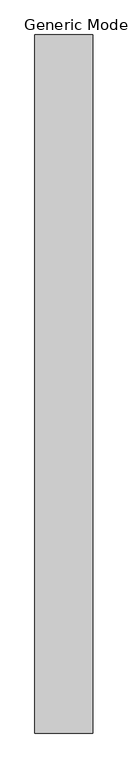
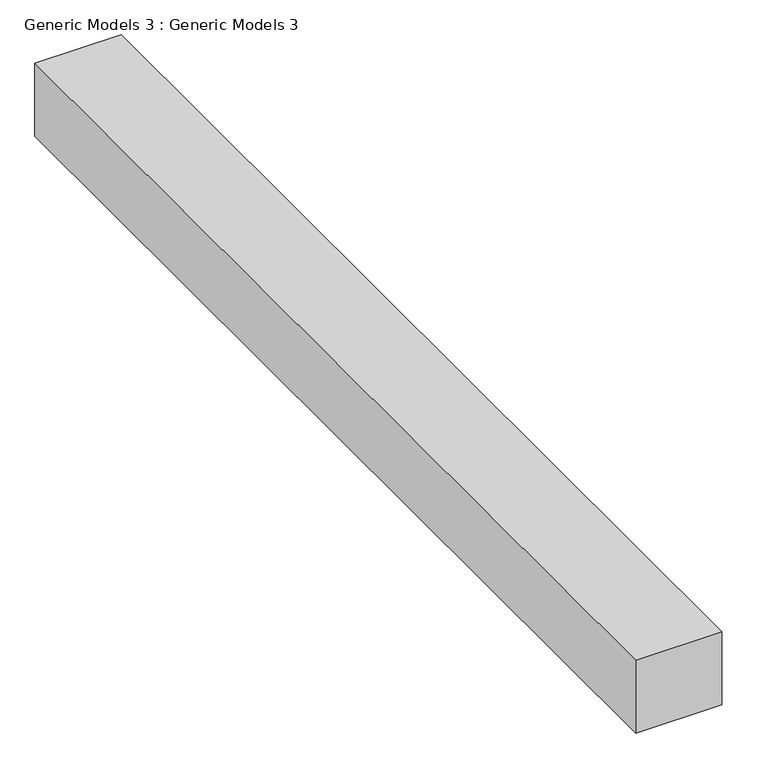
"""IFC4 building model written with IfcOpenShell, lengths in millimetres: proxy geometry, Generic Models 3 : Generic Models 3."""

from ifc_helpers import new_model, si_unit, frame, origin, place, context, project, spatial, polyline, outline, extrude, source, transform, mapped, element, save


def generic_models_3_generic_models_3_7314e451(model_context):
    return source(origin(), model_context, "Body", "SweptSolid", [
        extrude(outline(polyline([(-8586.8607234, -9739.3538163), (-8245.991855, -9739.3538163), (-8245.991855, -13854.1538163), (-8586.8607234, -13854.1538163), (-8586.8607234, -9739.3538163)])), frame((0.0, 0.0, 3352.8), z_axis=(0.0, 0.0, 1.0), x_axis=(1.0, 0.0, 0.0)), (0.0, 0.0, 1.0), 304.8),
    ])


if __name__ == "__main__":
    model = new_model("IFC4")
    model_context = context("Model", 3, world=origin())
    ifc_project = project(units=[si_unit("LENGTHUNIT", "METRE", prefix="MILLI")], contexts=[model_context])
    site = spatial("IfcSite", under=ifc_project)
    building = spatial("IfcBuilding", under=site)
    placement = place(None, origin())
    generic_models_3_generic_models_3_shape = generic_models_3_generic_models_3_7314e451(model_context)
    element("IfcBuildingElementProxy", 1, Name="Generic Models 3 : Generic Models 3", ObjectType="Generic Models 3 : Generic Models 3", at=placement, inside=building, context=model_context, shape_type="MappedRepresentation", body=[
        mapped(generic_models_3_generic_models_3_shape, transform((0.0, 0.0, 0.0), x_axis=(1.0, 0.0, 0.0), y_axis=(0.0, 1.0, 0.0), z_axis=(0.0, 0.0, 1.0))),
    ])
    save(model, "model.ifc")
